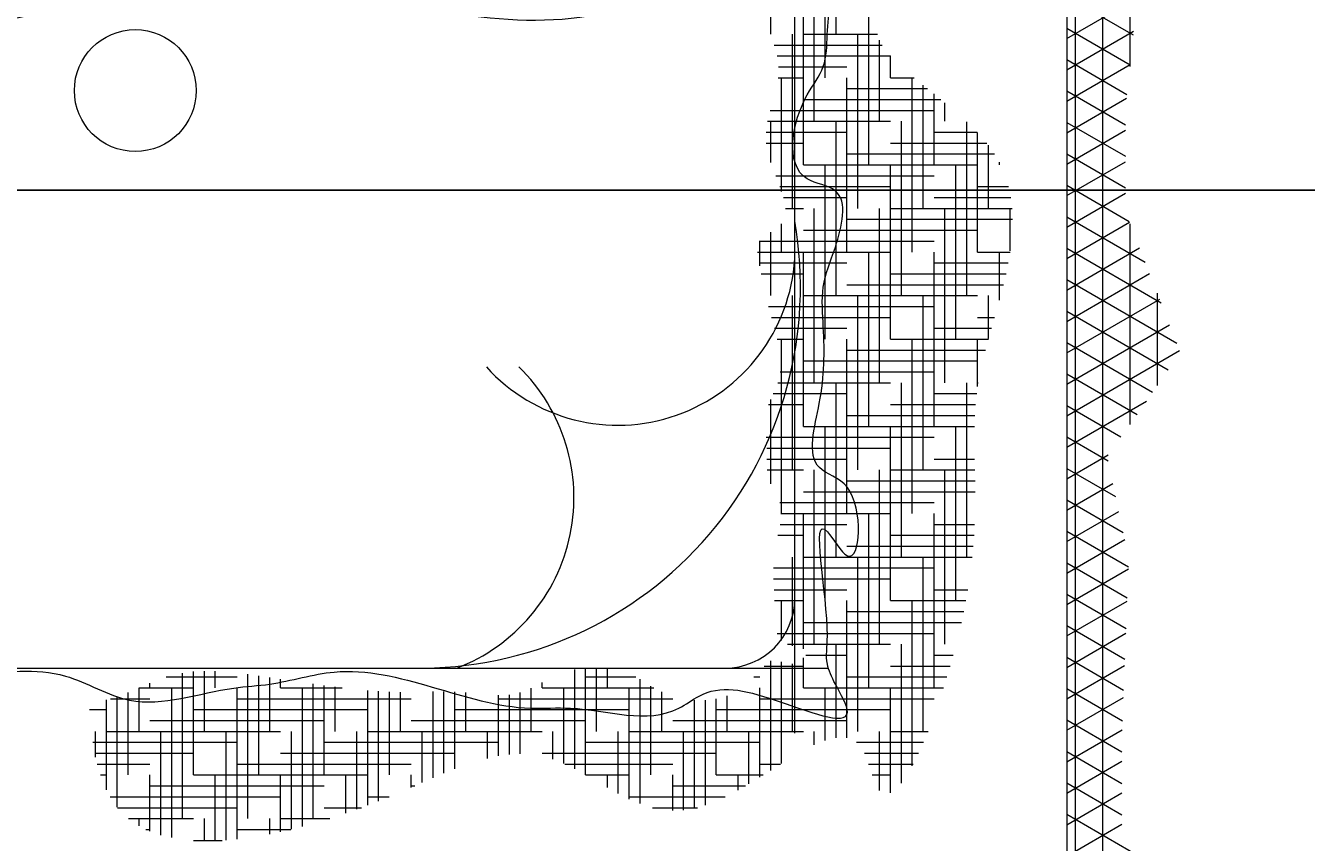
# Model space of a CAD drawing. Units: inches. Extents: x 3731 to 4318, y 1310 to 2388.
# Tile 27 of 57: x 3894 to 3954, y 1844 to 1882. Entities that reach past the tile are written whole.
import ezdxf

# ---------------------------------------------------------------- set-up
doc = ezdxf.new("R2010")
doc.units = ezdxf.units.IN
doc.layers.add('A-ANNO-DIMS', color=2, linetype='Continuous', lineweight=18)
doc.layers.add('A-FURN', color=8, linetype='Continuous', lineweight=13)
doc.styles.get("Standard").update_dxf_attribs({"font": 'arial.ttf'})
doc.dimstyles.get("Standard").update_dxf_attribs({"dimtxt": 0.18, "dimasz": 0.18, "dimexe": 0.18, "dimexo": 0.0625, "dimgap": 0.09, "dimtad": 0, "dimtih": 1, "dimtoh": 1, "dimdec": 4, "dimzin": 0, "dimdsep": 46, "dimtxsty": 'Standard', "dimcen": 0.09, "dimadec": 0, "dimazin": 0, "dimtfac": 1, "dimtdec": 4, "dimtofl": 0, "dimtmove": 0, "dimatfit": 3, "dimfxl": 1, "dimtolj": 1, "dimtzin": 0, "dimarcsym": 0})

# ---------------------------------------------------------------- blocks, each defined once
blk = doc.blocks.new('A$C200C7901')
at = {"linetype": 'ByBlock'}
for p, q in [((2.3224, 0.0468), (2.3224, 1.6627)), ((2.3224, 0.0468), (2.3224, 1.6627)), ((2.3537, 0.0056), (2.3537, 1.634)), ((2.3537, 0.0056), (2.3537, 1.634)), ((2.0474, 1.0977), (2.0474, 1.2977)), ((2.0474, 1.0977), (2.0474, 1.2977)), ((2.3849, 1.0607), (2.3849, 1.3013)), ((2.3849, 1.0607), (2.3849, 1.3013)), ((1.9724, 1.0977), (1.9724, 1.2927)), ((1.9724, 1.0977), (1.9724, 1.2927)), ((2.0349, 1.0477), (2.0349, 1.2477)), ((2.0349, 1.0477), (2.0349, 1.2477)), ((2.0099, 0.9477), (2.0099, 1.1477)), ((2.0099, 0.9477), (2.0099, 1.1477)), ((2.0849, 0.9477), (2.0849, 1.1477)), ((2.0849, 0.9477), (2.0849, 1.1477)), ((2.3121, 1.1408), (2.3884, 1.0967)), ((2.3121, 1.1408), (2.3884, 1.0967)), ((2.3121, 1.0928), (2.3915, 1.1386)), ((2.3121, 1.0928), (2.3915, 1.1386)), ((2.3121, 1.1047), (2.3851, 1.0625)), ((2.3121, 1.1047), (2.3851, 1.0625)), ((1.9974, 0.8977), (1.9974, 1.0977)), ((1.9974, 0.8977), (1.9974, 1.0977)), ((2.0099, 1.0977), (2.095, 1.0977)), ((2.0099, 1.0977), (2.095, 1.0977)), ((2.0724, 0.8977), (2.0724, 1.0977)), ((2.0724, 0.8977), (2.0724, 1.0977)), ((2.0974, 0.9977), (2.0974, 1.0909)), ((2.0974, 0.9977), (2.0974, 1.0909)), ((2.3121, 1.0567), (2.3887, 1.1009)), ((2.3121, 1.0567), (2.3887, 1.1009)), ((1.9763, 1.0852), (2.1005, 1.0852)), ((1.9763, 1.0852), (2.1005, 1.0852)), ((1.9799, 1.0727), (2.1099, 1.0727)), ((1.9799, 1.0727), (2.1099, 1.0727)), ((1.9815, 1.0602), (2.0599, 1.0602)), ((1.9815, 1.0602), (2.0599, 1.0602)), ((2.1099, 1.0477), (2.1099, 1.0729)), ((2.1099, 1.0477), (2.1099, 1.0729)), ((2.3121, 1.0686), (2.3813, 1.0286)), ((2.3121, 1.0686), (2.3813, 1.0286)), ((2.3121, 1.0206), (2.3851, 1.0628)), ((2.3121, 1.0206), (2.3851, 1.0628)), ((1.981, 1.0477), (2.0099, 1.0477)), ((1.981, 1.0477), (2.0099, 1.0477)), ((1.9849, 0.9171), (1.9849, 1.0477)), ((1.9849, 0.9171), (1.9849, 1.0477)), ((2.0599, 0.8477), (2.0599, 1.0477)), ((2.0599, 0.8477), (2.0599, 1.0477)), ((2.1099, 1.0477), (2.137, 1.0477)), ((2.1099, 1.0477), (2.137, 1.0477)), ((2.1349, 0.8477), (2.1349, 1.0477)), ((2.1349, 0.8477), (2.1349, 1.0477)), ((2.0599, 1.0352), (2.1523, 1.0352)), ((2.0599, 1.0352), (2.1523, 1.0352)), ((2.1474, 0.8977), (2.1474, 1.0391)), ((2.1474, 0.8977), (2.1474, 1.0391)), ((2.1599, 0.9477), (2.1599, 1.029)), ((2.1599, 0.9477), (2.1599, 1.029)), ((2.3121, 1.0325), (2.3795, 0.9936)), ((2.3121, 1.0325), (2.3795, 0.9936)), ((2.0099, 1.0227), (2.1678, 1.0227)), ((2.0099, 1.0227), (2.1678, 1.0227)), ((2.1724, 0.9977), (2.1724, 1.0189)), ((2.1724, 0.9977), (2.1724, 1.0189)), ((2.3121, 0.9846), (2.3809, 1.0242)), ((2.3121, 0.9846), (2.3809, 1.0242)), ((1.9718, 1.0102), (2.1599, 1.0102)), ((1.9718, 1.0102), (2.1599, 1.0102)), ((1.9671, 0.9852), (2.0599, 0.9852)), ((1.9671, 0.9852), (2.0599, 0.9852)), ((1.9688, 0.9977), (2.1099, 0.9977)), ((1.9688, 0.9977), (2.1099, 0.9977)), ((1.9724, 0.9504), (1.9724, 0.9977)), ((1.9724, 0.9504), (1.9724, 0.9977)), ((2.0474, 0.7977), (2.0474, 0.9977)), ((2.0474, 0.7977), (2.0474, 0.9977)), ((2.1224, 0.7977), (2.1224, 0.9977)), ((2.1224, 0.7977), (2.1224, 0.9977)), ((2.1599, 0.9852), (2.2095, 0.9852)), ((2.1599, 0.9852), (2.2095, 0.9852)), ((2.1974, 0.7977), (2.1974, 0.9972)), ((2.1974, 0.7977), (2.1974, 0.9972)), ((2.3121, 0.9964), (2.3795, 0.9575)), ((2.3121, 0.9964), (2.3795, 0.9575)), ((2.3121, 0.9485), (2.3795, 0.9874)), ((2.3121, 0.9485), (2.3795, 0.9874)), ((1.9672, 0.9727), (2.0099, 0.9727)), ((1.9672, 0.9727), (2.0099, 0.9727)), ((2.1099, 0.9727), (2.2204, 0.9727)), ((2.1099, 0.9727), (2.2204, 0.9727)), ((2.2099, 0.8477), (2.2099, 0.9848)), ((2.2099, 0.8477), (2.2099, 0.9848)), ((2.0599, 0.9602), (2.2294, 0.9602)), ((2.0599, 0.9602), (2.2294, 0.9602)), ((2.2224, 0.8977), (2.2224, 0.9702)), ((2.2224, 0.8977), (2.2224, 0.9702)), ((2.3121, 0.9603), (2.3795, 0.9215)), ((2.3121, 0.9603), (2.3795, 0.9215)), ((2.0099, 0.9477), (2.2099, 0.9477)), ((2.0099, 0.9477), (2.2099, 0.9477)), ((2.0349, 0.7477), (2.0349, 0.9477)), ((2.0349, 0.7477), (2.0349, 0.9477)), ((2.1099, 0.7477), (2.1099, 0.9477)), ((2.1099, 0.7477), (2.1099, 0.9477)), ((2.1849, 0.7477), (2.1849, 0.9477)), ((2.1849, 0.7477), (2.1849, 0.9477)), ((2.2349, 0.9477), (2.2349, 0.9506)), ((2.2349, 0.9477), (2.2349, 0.9506)), ((2.3121, 0.9124), (2.3795, 0.9513)), ((2.3121, 0.9124), (2.3795, 0.9513)), ((1.9781, 0.9352), (2.1599, 0.9352)), ((1.9781, 0.9352), (2.1599, 0.9352)), ((1.9829, 0.9227), (2.1099, 0.9227)), ((1.9829, 0.9227), (2.1099, 0.9227)), ((2.2099, 0.9227), (2.2455, 0.9227)), ((2.2099, 0.9227), (2.2455, 0.9227)), ((2.3121, 0.9243), (2.3838, 0.8829)), ((2.3121, 0.9243), (2.3838, 0.8829)), ((2.3121, 0.8763), (2.3795, 0.9152)), ((2.3121, 0.8763), (2.3795, 0.9152)), ((1.9871, 0.9102), (2.0599, 0.9102)), ((1.9871, 0.9102), (2.0599, 0.9102)), ((1.9894, 0.8977), (2.0099, 0.8977)), ((1.9894, 0.8977), (2.0099, 0.8977)), ((2.0224, 0.6977), (2.0224, 0.8977)), ((2.0224, 0.6977), (2.0224, 0.8977)), ((2.0974, 0.6977), (2.0974, 0.8977)), ((2.0974, 0.6977), (2.0974, 0.8977)), ((2.1099, 0.8977), (2.2496, 0.8977)), ((2.1099, 0.8977), (2.2496, 0.8977)), ((2.1599, 0.9102), (2.2481, 0.9102)), ((2.1599, 0.9102), (2.2481, 0.9102)), ((2.1724, 0.6977), (2.1724, 0.8977)), ((2.1724, 0.6977), (2.1724, 0.8977)), ((2.2474, 0.8489), (2.2474, 0.8977)), ((2.2474, 0.8489), (2.2474, 0.8977)), ((2.0599, 0.8852), (2.2501, 0.8852)), ((2.0599, 0.8852), (2.2501, 0.8852)), ((2.3121, 0.8882), (2.4022, 0.8362)), ((2.3121, 0.8882), (2.4022, 0.8362)), ((1.9724, 0.7977), (1.9724, 0.8703)), ((1.9724, 0.7977), (1.9724, 0.8703)), ((1.9849, 0.8477), (1.9849, 0.88)), ((1.9849, 0.8477), (1.9849, 0.88)), ((2.0099, 0.8727), (2.2099, 0.8727)), ((2.0099, 0.8727), (2.2099, 0.8727)), ((2.3121, 0.8402), (2.3842, 0.8818)), ((2.3121, 0.8402), (2.3842, 0.8818)), ((2.3849, 0.6497), (2.3849, 0.8801)), ((2.3849, 0.6497), (2.3849, 0.8801)), ((1.9599, 0.8317), (1.9599, 0.8604)), ((1.9599, 0.8317), (1.9599, 0.8604)), ((1.9599, 0.8602), (2.1599, 0.8602)), ((1.9599, 0.8602), (2.1599, 0.8602)), ((1.9574, 0.8477), (2.1099, 0.8477)), ((1.9574, 0.8477), (2.1099, 0.8477)), ((2.0099, 0.6477), (2.0099, 0.8477)), ((2.0099, 0.6477), (2.0099, 0.8477)), ((2.0849, 0.6477), (2.0849, 0.8477)), ((2.0849, 0.6477), (2.0849, 0.8477)), ((2.1599, 0.6477), (2.1599, 0.8477)), ((2.1599, 0.6477), (2.1599, 0.8477)), ((2.2099, 0.8477), (2.2472, 0.8477)), ((2.2099, 0.8477), (2.2472, 0.8477)), ((2.2349, 0.7923), (2.2349, 0.8477)), ((2.2349, 0.7923), (2.2349, 0.8477)), ((2.3121, 0.8041), (2.3958, 0.8524)), ((2.3121, 0.8041), (2.3958, 0.8524)), ((2.3121, 0.8521), (2.4205, 0.7895)), ((2.3121, 0.8521), (2.4205, 0.7895)), ((1.9593, 0.8352), (2.0599, 0.8352)), ((1.9593, 0.8352), (2.0599, 0.8352)), ((2.1599, 0.8352), (2.2451, 0.8352)), ((2.1599, 0.8352), (2.2451, 0.8352)), ((1.9615, 0.8227), (2.0099, 0.8227)), ((1.9615, 0.8227), (2.0099, 0.8227)), ((2.0599, 0.8102), (2.2396, 0.8102)), ((2.0599, 0.8102), (2.2396, 0.8102)), ((2.1099, 0.8227), (2.2425, 0.8227)), ((2.1099, 0.8227), (2.2425, 0.8227)), ((2.3121, 0.7681), (2.4073, 0.823)), ((2.3121, 0.7681), (2.4073, 0.823)), ((2.3121, 0.816), (2.4384, 0.7431)), ((2.3121, 0.816), (2.4384, 0.7431)), ((2.0099, 0.7977), (2.2099, 0.7977)), ((2.0099, 0.7977), (2.2099, 0.7977)), ((2.2224, 0.7483), (2.2224, 0.7977)), ((2.2224, 0.7483), (2.2224, 0.7977)), ((2.4162, 0.6946), (2.4162, 0.8006)), ((2.4162, 0.6946), (2.4162, 0.8006)), ((1.9699, 0.7852), (2.1599, 0.7852)), ((1.9699, 0.7852), (2.1599, 0.7852)), ((2.3121, 0.732), (2.4189, 0.7936)), ((2.3121, 0.732), (2.4189, 0.7936)), ((2.3121, 0.7799), (2.4287, 0.7126)), ((2.3121, 0.7799), (2.4287, 0.7126)), ((1.9734, 0.7727), (2.1099, 0.7727)), ((1.9734, 0.7727), (2.1099, 0.7727)), ((2.2099, 0.7727), (2.2294, 0.7727)), ((2.2099, 0.7727), (2.2294, 0.7727)), ((1.9767, 0.7602), (2.0599, 0.7602)), ((1.9767, 0.7602), (2.0599, 0.7602)), ((2.1599, 0.7602), (2.2258, 0.7602)), ((2.1599, 0.7602), (2.2258, 0.7602)), ((2.3121, 0.6959), (2.4303, 0.7641)), ((2.3121, 0.6959), (2.4303, 0.7641)), ((1.9797, 0.7477), (2.0099, 0.7477)), ((1.9797, 0.7477), (2.0099, 0.7477)), ((2.0599, 0.7352), (2.2188, 0.7352)), ((2.0599, 0.7352), (2.2188, 0.7352)), ((2.1099, 0.7477), (2.2222, 0.7477)), ((2.1099, 0.7477), (2.2222, 0.7477)), ((2.2099, 0.6933), (2.2099, 0.7477)), ((2.2099, 0.6933), (2.2099, 0.7477)), ((2.3121, 0.7438), (2.4108, 0.6869)), ((2.3121, 0.7438), (2.4108, 0.6869)), ((2.0099, 0.7227), (2.2099, 0.7227)), ((2.0099, 0.7227), (2.2099, 0.7227)), ((2.3121, 0.6598), (2.4417, 0.7346)), ((2.3121, 0.6598), (2.4417, 0.7346)), ((1.9831, 0.7102), (2.1599, 0.7102)), ((1.9831, 0.7102), (2.1599, 0.7102)), ((2.3121, 0.7078), (2.3929, 0.6611)), ((2.3121, 0.7078), (2.3929, 0.6611)), ((1.9804, 0.6977), (2.1099, 0.6977)), ((1.9804, 0.6977), (2.1099, 0.6977)), ((2.0474, 0.4977), (2.0474, 0.6977)), ((2.0474, 0.4977), (2.0474, 0.6977)), ((2.1224, 0.4977), (2.1224, 0.6977)), ((2.1224, 0.4977), (2.1224, 0.6977)), ((2.1974, 0.4977), (2.1974, 0.6977)), ((2.1974, 0.4977), (2.1974, 0.6977)), ((2.2099, 0.6977), (2.2106, 0.6977)), ((2.2099, 0.6977), (2.2106, 0.6977)), ((1.9724, 0.5818), (1.9724, 0.6786)), ((1.9724, 0.5818), (1.9724, 0.6786)), ((1.9753, 0.6852), (2.0599, 0.6852)), ((1.9753, 0.6852), (2.0599, 0.6852)), ((2.1599, 0.6852), (2.2088, 0.6852)), ((2.1599, 0.6852), (2.2088, 0.6852)), ((2.3121, 0.6237), (2.4036, 0.6765)), ((2.3121, 0.6237), (2.4036, 0.6765)), ((1.97, 0.6727), (2.0099, 0.6727)), ((1.97, 0.6727), (2.0099, 0.6727)), ((2.1099, 0.6727), (2.2075, 0.6727)), ((2.1099, 0.6727), (2.2075, 0.6727)), ((2.3121, 0.6717), (2.3744, 0.6357)), ((2.3121, 0.6717), (2.3744, 0.6357)), ((2.0099, 0.6477), (2.2062, 0.6477)), ((2.0099, 0.6477), (2.2062, 0.6477)), ((2.0349, 0.4477), (2.0349, 0.6477)), ((2.0349, 0.4477), (2.0349, 0.6477)), ((2.0599, 0.6602), (2.2067, 0.6602)), ((2.0599, 0.6602), (2.2067, 0.6602)), ((2.1099, 0.4477), (2.1099, 0.6477)), ((2.1099, 0.4477), (2.1099, 0.6477)), ((2.1849, 0.4477), (2.1849, 0.6477)), ((2.1849, 0.4477), (2.1849, 0.6477)), ((1.9673, 0.6352), (2.1599, 0.6352)), ((1.9673, 0.6352), (2.1599, 0.6352)), ((2.3121, 0.6356), (2.3598, 0.6081)), ((2.3121, 0.6356), (2.3598, 0.6081)), ((1.9678, 0.6227), (2.1099, 0.6227)), ((1.9678, 0.6227), (2.1099, 0.6227)), ((1.9679, 0.6102), (2.0599, 0.6102)), ((1.9679, 0.6102), (2.0599, 0.6102)), ((2.1599, 0.6102), (2.2064, 0.6102)), ((2.1599, 0.6102), (2.2064, 0.6102)), ((2.3121, 0.5876), (2.3598, 0.6151)), ((2.3121, 0.5876), (2.3598, 0.6151)), ((1.9685, 0.5977), (2.0099, 0.5977)), ((1.9685, 0.5977), (2.0099, 0.5977)), ((2.0224, 0.3977), (2.0224, 0.5977)), ((2.0224, 0.3977), (2.0224, 0.5977)), ((2.0974, 0.3977), (2.0974, 0.5977)), ((2.0974, 0.3977), (2.0974, 0.5977)), ((2.1099, 0.5977), (2.2066, 0.5977)), ((2.1099, 0.5977), (2.2066, 0.5977)), ((2.1724, 0.3977), (2.1724, 0.5977)), ((2.1724, 0.3977), (2.1724, 0.5977)), ((2.3121, 0.5995), (2.3682, 0.5671)), ((2.3121, 0.5995), (2.3682, 0.5671)), ((2.0599, 0.5852), (2.2069, 0.5852)), ((2.0599, 0.5852), (2.2069, 0.5852)), ((2.3121, 0.5515), (2.365, 0.5821)), ((2.3121, 0.5515), (2.365, 0.5821)), ((1.9827, 0.5602), (2.1599, 0.5602)), ((1.9827, 0.5602), (2.1599, 0.5602)), ((2.0099, 0.5727), (2.207, 0.5727)), ((2.0099, 0.5727), (2.207, 0.5727)), ((2.3121, 0.5634), (2.3771, 0.5259)), ((2.3121, 0.5634), (2.3771, 0.5259)), ((1.9842, 0.5477), (2.1099, 0.5477)), ((1.9842, 0.5477), (2.1099, 0.5477)), ((2.0099, 0.3923), (2.0099, 0.5477)), ((2.0099, 0.3923), (2.0099, 0.5477)), ((2.0849, 0.3477), (2.0849, 0.5477)), ((2.0849, 0.3477), (2.0849, 0.5477)), ((2.1599, 0.3477), (2.1599, 0.5477)), ((2.1599, 0.3477), (2.1599, 0.5477)), ((2.3121, 0.5155), (2.3719, 0.55)), ((2.3121, 0.5155), (2.3719, 0.55)), ((1.9831, 0.5352), (2.0599, 0.5352)), ((1.9831, 0.5352), (2.0599, 0.5352)), ((2.1599, 0.5352), (2.2065, 0.5352)), ((2.1599, 0.5352), (2.2065, 0.5352)), ((1.9807, 0.5227), (2.0099, 0.5227)), ((1.9807, 0.5227), (2.0099, 0.5227)), ((2.1099, 0.5227), (2.2058, 0.5227)), ((2.1099, 0.5227), (2.2058, 0.5227)), ((2.3121, 0.5273), (2.383, 0.4864)), ((2.3121, 0.5273), (2.383, 0.4864)), ((2.3121, 0.4794), (2.3788, 0.5179)), ((2.3121, 0.4794), (2.3788, 0.5179)), ((2.0599, 0.5102), (2.2049, 0.5102)), ((2.0599, 0.5102), (2.2049, 0.5102)), ((1.9755, 0.4852), (2.1599, 0.4852)), ((1.9755, 0.4852), (2.1599, 0.4852)), ((1.9974, 0.3957), (1.9974, 0.4977)), ((1.9974, 0.3957), (1.9974, 0.4977)), ((2.0099, 0.4977), (2.2038, 0.4977)), ((2.0099, 0.4977), (2.2038, 0.4977)), ((2.0724, 0.2977), (2.0724, 0.4977)), ((2.0724, 0.2977), (2.0724, 0.4977)), ((2.1474, 0.2977), (2.1474, 0.4977)), ((2.1474, 0.2977), (2.1474, 0.4977)), ((2.3121, 0.4912), (2.3817, 0.4511)), ((2.3121, 0.4912), (2.3817, 0.4511)), ((1.9757, 0.4727), (2.1099, 0.4727)), ((1.9757, 0.4727), (2.1099, 0.4727)), ((2.3121, 0.4433), (2.383, 0.4842)), ((2.3121, 0.4433), (2.383, 0.4842)), ((1.9762, 0.4602), (2.0599, 0.4602)), ((1.9762, 0.4602), (2.0599, 0.4602)), ((2.1599, 0.4602), (2.1987, 0.4602)), ((2.1599, 0.4602), (2.1987, 0.4602)), ((1.9768, 0.4477), (2.0099, 0.4477)), ((1.9768, 0.4477), (2.0099, 0.4477)), ((1.9849, 0.402), (1.9849, 0.4477)), ((1.9849, 0.402), (1.9849, 0.4477)), ((2.0599, 0.2903), (2.0599, 0.4477)), ((2.0599, 0.2903), (2.0599, 0.4477)), ((2.1099, 0.4477), (2.1965, 0.4477)), ((2.1099, 0.4477), (2.1965, 0.4477)), ((2.1349, 0.2582), (2.1349, 0.4477)), ((2.1349, 0.2582), (2.1349, 0.4477)), ((2.3121, 0.4552), (2.3803, 0.4158)), ((2.3121, 0.4552), (2.3803, 0.4158)), ((2.3121, 0.4072), (2.3815, 0.4473)), ((2.3121, 0.4072), (2.3815, 0.4473)), ((2.0599, 0.4352), (2.194, 0.4352)), ((2.0599, 0.4352), (2.194, 0.4352)), ((2.0099, 0.4227), (2.1913, 0.4227)), ((2.0099, 0.4227), (2.1913, 0.4227)), ((2.3121, 0.4191), (2.3789, 0.3805)), ((2.3121, 0.4191), (2.3789, 0.3805)), ((1.9797, 0.4102), (2.1599, 0.4102)), ((1.9797, 0.4102), (2.1599, 0.4102)), ((1.9915, 0.3977), (2.1099, 0.3977)), ((1.9915, 0.3977), (2.1099, 0.3977)), ((2.0474, 0.2905), (2.0474, 0.3977)), ((2.0474, 0.2905), (2.0474, 0.3977)), ((2.1224, 0.2385), (2.1224, 0.3977)), ((2.1224, 0.2385), (2.1224, 0.3977)), ((2.3121, 0.3711), (2.3801, 0.4103)), ((2.3121, 0.3711), (2.3801, 0.4103)), ((2.0127, 0.3852), (2.0599, 0.3852)), ((2.0127, 0.3852), (2.0599, 0.3852)), ((2.1599, 0.3852), (2.1819, 0.3852)), ((2.1599, 0.3852), (2.1819, 0.3852)), ((2.3121, 0.383), (2.3775, 0.3452)), ((2.3121, 0.383), (2.3775, 0.3452)), ((1.7474, 0.2546), (1.7474, 0.3689)), ((1.7474, 0.2546), (1.7474, 0.3689)), ((1.7599, 0.2477), (1.7599, 0.3703)), ((1.7599, 0.2477), (1.7599, 0.3703)), ((1.7724, 0.2977), (1.7724, 0.3703)), ((1.7724, 0.2977), (1.7724, 0.3703)), ((1.7849, 0.3477), (1.7849, 0.3703)), ((1.7849, 0.3477), (1.7849, 0.3703)), ((1.9648, 0.3727), (2.0099, 0.3727)), ((1.9648, 0.3727), (2.0099, 0.3727)), ((1.9724, 0.253), (1.9724, 0.3785)), ((1.9724, 0.253), (1.9724, 0.3785)), ((1.9849, 0.2609), (1.9849, 0.3774)), ((1.9849, 0.2609), (1.9849, 0.3774)), ((1.9974, 0.2977), (1.9974, 0.3753)), ((1.9974, 0.2977), (1.9974, 0.3753)), ((2.0099, 0.3477), (2.0099, 0.382)), ((2.0099, 0.3477), (2.0099, 0.382)), ((2.1099, 0.3727), (2.1784, 0.3727)), ((2.1099, 0.3727), (2.1784, 0.3727)), ((2.3121, 0.335), (2.3786, 0.3734)), ((2.3121, 0.335), (2.3786, 0.3734)), ((1.2599, 0.3477), (1.2599, 0.3531)), ((1.2599, 0.3477), (1.2599, 0.3531)), ((1.2785, 0.3602), (1.3599, 0.3602)), ((1.2785, 0.3602), (1.3599, 0.3602)), ((1.2974, 0.1977), (1.2974, 0.3647)), ((1.2974, 0.1977), (1.2974, 0.3647)), ((1.3099, 0.2477), (1.3099, 0.3663)), ((1.3099, 0.2477), (1.3099, 0.3663)), ((1.3224, 0.2977), (1.3224, 0.3669)), ((1.3224, 0.2977), (1.3224, 0.3669)), ((1.3349, 0.3477), (1.3349, 0.3668)), ((1.3349, 0.3477), (1.3349, 0.3668)), ((1.3724, 0.1977), (1.3724, 0.3634)), ((1.3724, 0.1977), (1.3724, 0.3634)), ((1.3849, 0.2477), (1.3849, 0.3616)), ((1.3849, 0.2477), (1.3849, 0.3616)), ((1.3974, 0.2977), (1.3974, 0.3597)), ((1.3974, 0.2977), (1.3974, 0.3597)), ((1.4099, 0.3477), (1.4099, 0.3578)), ((1.4099, 0.3477), (1.4099, 0.3578)), ((1.7099, 0.3477), (1.7099, 0.3539)), ((1.7099, 0.3477), (1.7099, 0.3539)), ((1.7599, 0.3602), (1.8177, 0.3602)), ((1.7599, 0.3602), (1.8177, 0.3602)), ((1.8224, 0.2148), (1.8224, 0.3575)), ((1.8224, 0.2148), (1.8224, 0.3575)), ((1.9532, 0.3602), (1.9599, 0.3602)), ((1.9532, 0.3602), (1.9599, 0.3602)), ((2.0599, 0.3602), (2.1747, 0.3602)), ((2.0599, 0.3602), (2.1747, 0.3602)), ((1.2349, 0.2477), (1.2349, 0.3422)), ((1.2349, 0.2477), (1.2349, 0.3422)), ((1.2474, 0.2977), (1.2474, 0.3476)), ((1.2474, 0.2977), (1.2474, 0.3476)), ((1.2475, 0.3477), (1.3099, 0.3477)), ((1.2475, 0.3477), (1.3099, 0.3477)), ((1.2849, 0.1758), (1.2849, 0.3477)), ((1.2849, 0.1758), (1.2849, 0.3477)), ((1.3599, 0.1741), (1.3599, 0.3477)), ((1.3599, 0.1741), (1.3599, 0.3477)), ((1.4099, 0.3477), (1.4806, 0.3477)), ((1.4099, 0.3477), (1.4806, 0.3477)), ((1.4349, 0.1886), (1.4349, 0.3477)), ((1.4349, 0.1886), (1.4349, 0.3477)), ((1.4474, 0.1977), (1.4474, 0.3521)), ((1.4474, 0.1977), (1.4474, 0.3521)), ((1.4599, 0.2477), (1.4599, 0.3504)), ((1.4599, 0.2477), (1.4599, 0.3504)), ((1.4724, 0.2977), (1.4724, 0.3487)), ((1.4724, 0.2977), (1.4724, 0.3487)), ((1.5099, 0.2129), (1.5099, 0.3447)), ((1.5099, 0.2129), (1.5099, 0.3447)), ((1.5224, 0.2177), (1.5224, 0.3438)), ((1.5224, 0.2177), (1.5224, 0.3438)), ((1.5349, 0.2477), (1.5349, 0.3431)), ((1.5349, 0.2477), (1.5349, 0.3431)), ((1.5474, 0.2977), (1.5474, 0.3428)), ((1.5474, 0.2977), (1.5474, 0.3428)), ((1.5849, 0.2443), (1.5849, 0.3434)), ((1.5849, 0.2443), (1.5849, 0.3434)), ((1.5974, 0.2496), (1.5974, 0.3435)), ((1.5974, 0.2496), (1.5974, 0.3435)), ((1.6099, 0.2546), (1.6099, 0.3432)), ((1.6099, 0.2546), (1.6099, 0.3432)), ((1.6224, 0.2977), (1.6224, 0.3424)), ((1.6224, 0.2977), (1.6224, 0.3424)), ((1.6599, 0.2695), (1.6599, 0.3394)), ((1.6599, 0.2695), (1.6599, 0.3394)), ((1.6724, 0.2713), (1.6724, 0.3398)), ((1.6724, 0.2713), (1.6724, 0.3398)), ((1.6849, 0.272), (1.6849, 0.3422)), ((1.6849, 0.272), (1.6849, 0.3422)), ((1.6974, 0.2977), (1.6974, 0.3472)), ((1.6974, 0.2977), (1.6974, 0.3472)), ((1.7099, 0.3477), (1.8383, 0.3477)), ((1.7099, 0.3477), (1.8383, 0.3477)), ((1.7349, 0.2607), (1.7349, 0.3477)), ((1.7349, 0.2607), (1.7349, 0.3477)), ((1.8099, 0.2201), (1.8099, 0.3477)), ((1.8099, 0.2201), (1.8099, 0.3477)), ((1.8349, 0.2477), (1.8349, 0.3497)), ((1.8349, 0.2477), (1.8349, 0.3497)), ((1.8474, 0.2977), (1.8474, 0.3432)), ((1.8474, 0.2977), (1.8474, 0.3432)), ((1.9224, 0.2977), (1.9224, 0.3385)), ((1.9224, 0.2977), (1.9224, 0.3385)), ((1.9599, 0.2452), (1.9599, 0.3477)), ((1.9599, 0.2452), (1.9599, 0.3477)), ((2.0099, 0.3477), (2.1708, 0.3477)), ((2.0099, 0.3477), (2.1708, 0.3477)), ((2.0349, 0.2874), (2.0349, 0.3477)), ((2.0349, 0.2874), (2.0349, 0.3477)), ((2.1099, 0.2274), (2.1099, 0.3477)), ((2.1099, 0.2274), (2.1099, 0.3477)), ((2.3121, 0.3469), (2.3761, 0.31)), ((2.3121, 0.3469), (2.3761, 0.31)), ((1.2099, 0.2308), (1.2099, 0.334)), ((1.2099, 0.2308), (1.2099, 0.334)), ((1.2148, 0.3352), (1.2599, 0.3352)), ((1.2148, 0.3352), (1.2599, 0.3352)), ((1.2224, 0.2106), (1.2224, 0.3375)), ((1.2224, 0.2106), (1.2224, 0.3375)), ((1.3599, 0.3352), (1.5599, 0.3352)), ((1.3599, 0.3352), (1.5599, 0.3352)), ((1.6599, 0.3352), (1.8599, 0.3352)), ((1.6599, 0.3352), (1.8599, 0.3352)), ((1.8849, 0.2093), (1.8849, 0.3337)), ((1.8849, 0.2093), (1.8849, 0.3337)), ((1.8974, 0.2129), (1.8974, 0.3335)), ((1.8974, 0.2129), (1.8974, 0.3335)), ((1.9099, 0.2477), (1.9099, 0.3349)), ((1.9099, 0.2477), (1.9099, 0.3349)), ((1.9599, 0.3352), (2.1599, 0.3352)), ((1.9599, 0.3352), (2.1599, 0.3352)), ((2.3121, 0.299), (2.3772, 0.3365)), ((2.3121, 0.299), (2.3772, 0.3365)), ((1.1904, 0.3227), (1.2099, 0.3227)), ((1.1904, 0.3227), (1.2099, 0.3227)), ((1.2599, 0.3102), (1.4599, 0.3102)), ((1.2599, 0.3102), (1.4599, 0.3102)), ((1.3099, 0.3227), (1.5099, 0.3227)), ((1.3099, 0.3227), (1.5099, 0.3227)), ((1.5599, 0.3102), (1.7599, 0.3102)), ((1.5599, 0.3102), (1.7599, 0.3102)), ((1.6099, 0.3227), (1.8099, 0.3227)), ((1.6099, 0.3227), (1.8099, 0.3227)), ((1.8599, 0.3102), (2.0599, 0.3102)), ((1.8599, 0.3102), (2.0599, 0.3102)), ((1.9099, 0.3227), (2.1099, 0.3227)), ((1.9099, 0.3227), (2.1099, 0.3227)), ((2.3121, 0.3108), (2.3755, 0.2742)), ((2.3121, 0.3108), (2.3755, 0.2742)), ((1.1974, 0.2683), (1.1974, 0.2977)), ((1.1974, 0.2683), (1.1974, 0.2977)), ((1.2099, 0.2977), (1.4099, 0.2977)), ((1.2099, 0.2977), (1.4099, 0.2977)), ((1.2724, 0.1788), (1.2724, 0.2977)), ((1.2724, 0.1788), (1.2724, 0.2977)), ((1.3474, 0.173), (1.3474, 0.2977)), ((1.3474, 0.173), (1.3474, 0.2977)), ((1.4224, 0.1854), (1.4224, 0.2977)), ((1.4224, 0.1854), (1.4224, 0.2977)), ((1.4974, 0.2083), (1.4974, 0.2977)), ((1.4974, 0.2083), (1.4974, 0.2977)), ((1.5099, 0.2977), (1.7099, 0.2977)), ((1.5099, 0.2977), (1.7099, 0.2977)), ((1.5724, 0.2389), (1.5724, 0.2977)), ((1.5724, 0.2389), (1.5724, 0.2977)), ((1.6474, 0.2668), (1.6474, 0.2977)), ((1.6474, 0.2668), (1.6474, 0.2977)), ((1.7224, 0.2658), (1.7224, 0.2977)), ((1.7224, 0.2658), (1.7224, 0.2977)), ((1.7974, 0.2263), (1.7974, 0.2977)), ((1.7974, 0.2263), (1.7974, 0.2977)), ((1.8099, 0.2977), (2.0099, 0.2977)), ((1.8099, 0.2977), (2.0099, 0.2977)), ((1.8724, 0.2072), (1.8724, 0.2977)), ((1.8724, 0.2072), (1.8724, 0.2977)), ((1.9474, 0.2376), (1.9474, 0.2977)), ((1.9474, 0.2376), (1.9474, 0.2977)), ((2.0224, 0.2822), (2.0224, 0.2977)), ((2.0224, 0.2822), (2.0224, 0.2977)), ((2.0974, 0.2299), (2.0974, 0.2977)), ((2.0974, 0.2299), (2.0974, 0.2977)), ((2.1099, 0.2977), (2.153, 0.2977)), ((2.1099, 0.2977), (2.153, 0.2977)), ((2.3121, 0.2629), (2.3757, 0.2996)), ((2.3121, 0.2629), (2.3757, 0.2996)), ((1.1943, 0.2852), (1.3599, 0.2852)), ((1.1943, 0.2852), (1.3599, 0.2852)), ((1.4599, 0.2852), (1.6599, 0.2852)), ((1.4599, 0.2852), (1.6599, 0.2852)), ((1.7599, 0.2852), (1.9599, 0.2852)), ((1.7599, 0.2852), (1.9599, 0.2852)), ((2.0708, 0.2852), (2.1478, 0.2852)), ((2.0708, 0.2852), (2.1478, 0.2852)), ((1.1965, 0.2727), (1.3099, 0.2727)), ((1.1965, 0.2727), (1.3099, 0.2727)), ((1.4099, 0.2727), (1.6099, 0.2727)), ((1.4099, 0.2727), (1.6099, 0.2727)), ((1.7099, 0.2727), (1.9099, 0.2727)), ((1.7099, 0.2727), (1.9099, 0.2727)), ((2.08, 0.2727), (2.1422, 0.2727)), ((2.08, 0.2727), (2.1422, 0.2727)), ((2.3121, 0.2747), (2.3755, 0.2381)), ((2.3121, 0.2747), (2.3755, 0.2381)), ((1.1994, 0.2602), (1.2599, 0.2602)), ((1.1994, 0.2602), (1.2599, 0.2602)), ((1.3599, 0.2602), (1.5599, 0.2602)), ((1.3599, 0.2602), (1.5599, 0.2602)), ((1.7361, 0.2602), (1.8599, 0.2602)), ((1.7361, 0.2602), (1.8599, 0.2602)), ((1.9599, 0.2602), (1.9838, 0.2602)), ((1.9599, 0.2602), (1.9838, 0.2602)), ((2.0848, 0.2602), (2.1359, 0.2602)), ((2.0848, 0.2602), (2.1359, 0.2602)), ((2.3121, 0.2268), (2.3755, 0.2634)), ((2.3121, 0.2268), (2.3755, 0.2634)), ((1.2031, 0.2477), (1.2099, 0.2477)), ((1.2031, 0.2477), (1.2099, 0.2477)), ((1.2599, 0.1831), (1.2599, 0.2477)), ((1.2599, 0.1831), (1.2599, 0.2477)), ((1.3099, 0.2477), (1.5099, 0.2477)), ((1.3099, 0.2477), (1.5099, 0.2477)), ((1.3349, 0.1723), (1.3349, 0.2477)), ((1.3349, 0.1723), (1.3349, 0.2477)), ((1.4099, 0.1825), (1.4099, 0.2477)), ((1.4099, 0.1825), (1.4099, 0.2477)), ((1.4849, 0.2039), (1.4849, 0.2477)), ((1.4849, 0.2039), (1.4849, 0.2477)), ((1.5599, 0.2335), (1.5599, 0.2477)), ((1.5599, 0.2335), (1.5599, 0.2477)), ((1.7599, 0.2477), (1.8099, 0.2477)), ((1.7599, 0.2477), (1.8099, 0.2477)), ((1.7849, 0.2332), (1.7849, 0.2477)), ((1.7849, 0.2332), (1.7849, 0.2477)), ((1.8599, 0.2068), (1.8599, 0.2477)), ((1.8599, 0.2068), (1.8599, 0.2477)), ((1.9099, 0.2477), (1.9639, 0.2477)), ((1.9099, 0.2477), (1.9639, 0.2477)), ((1.9349, 0.2304), (1.9349, 0.2477)), ((1.9349, 0.2304), (1.9349, 0.2477)), ((2.0888, 0.2477), (2.1099, 0.2477)), ((2.0888, 0.2477), (2.1099, 0.2477)), ((2.3121, 0.2387), (2.3755, 0.202)), ((2.3121, 0.2387), (2.3755, 0.202)), ((1.2142, 0.2227), (1.4099, 0.2227)), ((1.2142, 0.2227), (1.4099, 0.2227)), ((1.2599, 0.2352), (1.4599, 0.2352)), ((1.2599, 0.2352), (1.4599, 0.2352)), ((1.5099, 0.2227), (1.5346, 0.2227)), ((1.5099, 0.2227), (1.5346, 0.2227)), ((1.5599, 0.2352), (1.5638, 0.2352)), ((1.5599, 0.2352), (1.5638, 0.2352)), ((1.8099, 0.2227), (1.9203, 0.2227)), ((1.8099, 0.2227), (1.9203, 0.2227)), ((1.8599, 0.2352), (1.9433, 0.2352)), ((1.8599, 0.2352), (1.9433, 0.2352)), ((2.3121, 0.1907), (2.3755, 0.2273)), ((2.3121, 0.1907), (2.3755, 0.2273)), ((1.2227, 0.2102), (1.3599, 0.2102)), ((1.2227, 0.2102), (1.3599, 0.2102)), ((1.4599, 0.2102), (1.5027, 0.2102)), ((1.4599, 0.2102), (1.5027, 0.2102)), ((1.8368, 0.2102), (1.8884, 0.2102)), ((1.8368, 0.2102), (1.8884, 0.2102)), ((1.2351, 0.1977), (1.3099, 0.1977)), ((1.2351, 0.1977), (1.3099, 0.1977)), ((1.2474, 0.1892), (1.2474, 0.1977)), ((1.2474, 0.1892), (1.2474, 0.1977)), ((1.3224, 0.1722), (1.3224, 0.1977)), ((1.3224, 0.1722), (1.3224, 0.1977)), ((1.3974, 0.1799), (1.3974, 0.1977)), ((1.3974, 0.1799), (1.3974, 0.1977)), ((1.4099, 0.1977), (1.4662, 0.1977)), ((1.4099, 0.1977), (1.4662, 0.1977)), ((2.3121, 0.2026), (2.3953, 0.1545)), ((2.3121, 0.2026), (2.3953, 0.1545)), ((2.3121, 0.1546), (2.3755, 0.1912)), ((2.3121, 0.1546), (2.3755, 0.1912)), ((1.2552, 0.1852), (1.2599, 0.1852)), ((1.2552, 0.1852), (1.2599, 0.1852)), ((1.3599, 0.1852), (1.4215, 0.1852)), ((1.3599, 0.1852), (1.4215, 0.1852)), ((1.3099, 0.1727), (1.3428, 0.1727)), ((1.3099, 0.1727), (1.3428, 0.1727))]:
    blk.add_line(p, q, dxfattribs=at)
for p, q in [((2.3121, 1.6596), (2.3121, 0.0201)), ((2, 0.2957), (2, 1.2957)), ((2.0224, 0.9977), (2.0224, 1.1977)), ((2.0224, 0.9977), (2.0224, 1.1977)), ((1.9974, 0.5977), (1.9974, 0.7977)), ((1.9974, 0.5977), (1.9974, 0.7977)), ((2.0724, 0.5977), (2.0724, 0.7977)), ((2.0724, 0.5977), (2.0724, 0.7977)), ((2.1474, 0.5977), (2.1474, 0.7977)), ((2.1474, 0.5977), (2.1474, 0.7977)), ((1.9849, 0.5477), (1.9849, 0.7477)), ((1.9849, 0.5477), (1.9849, 0.7477)), ((2.0599, 0.5477), (2.0599, 0.7477)), ((2.0599, 0.5477), (2.0599, 0.7477)), ((2.1349, 0.5477), (2.1349, 0.7477)), ((2.1349, 0.5477), (2.1349, 0.7477)), ((0.4061, 0.3703), (2.0386, 0.3703))]:
    blk.add_line(p, q)
blk.add_circle((1.2431, 1.0329), 0.0699)
for centre, radius, start, end in [((1.5693, 0.8075), 0.4372, 269.0679, 9.9322), ((1.7969, 0.8525), 0.2035, 222.1514, 356.4639), ((1.5372, 0.5659), 0.2094, 290.9415, 45.7647), ((1.92, 0.4503), 0.08, 270, 0)]:
    blk.add_arc(centre, radius, start, end)
blk.add_open_spline([(0.4856, 1.3429), (0.5504, 1.3182), (0.6715, 1.2721), (0.8374, 1.0498), (1.1164, 1.1183), (1.3878, 1.1816), (1.5888, 1.1102), (1.8403, 1.1127), (1.9415, 1.2178), (2.0032, 1.2819)], degree=3, knots=[0, 0, 0, 0, 205.411753, 383.654933, 772.067458, 921.644661, 1226.793228, 1388.983508, 1642.292305, 1642.292305, 1642.292305, 1642.292305])
blk.add_open_spline([(0.473, 1.2954), (0.4739, 1.2781), (0.4755, 1.2477), (0.5032, 1.2084), (0.4801, 1.1701), (0.4928, 1.1255), (0.4674, 1.0912), (0.4579, 1.0351), (0.501, 0.9724), (0.4311, 0.8832), (0.4902, 0.8637), (0.4843, 0.8288), (0.4774, 0.7906), (0.4625, 0.7457), (0.459, 0.6999), (0.4816, 0.6664), (0.4748, 0.625), (0.4791, 0.5889), (0.4533, 0.5528), (0.4738, 0.5004), (0.4658, 0.4502), (0.4696, 0.3946), (0.4189, 0.3935), (0.4493, 0.3684), (0.4694, 0.3857), (0.4922, 0.3576), (0.5297, 0.3262), (0.5917, 0.3353), (0.6454, 0.3754), (0.7083, 0.3741), (0.7643, 0.3328), (0.826, 0.346), (0.925, 0.3388), (1.0353, 0.3593), (1.1561, 0.3744), (1.2477, 0.3154), (1.3302, 0.3474), (1.4086, 0.3512), (1.5217, 0.3878), (1.6362, 0.3176), (1.7682, 0.3285), (1.8402, 0.3019), (1.9071, 0.3529), (1.9647, 0.3412), (2.0795, 0.2948), (2.0472, 0.3498), (2.0343, 0.3772), (2.0435, 0.43), (2.0109, 0.5782), (2.0746, 0.4643), (2.0805, 0.584), (2.0084, 0.5979), (2.0343, 0.6846), (2.0344, 0.746), (2.0293, 0.8096), (2.0489, 0.8545), (2.0652, 0.9218), (1.9842, 0.9297), (2.0007, 1.0162), (2.0367, 1.0585), (2.0367, 1.1102), (2.0457, 1.1647), (2.0226, 1.2084), (2.0234, 1.2306), (2.0236, 1.2352)], degree=3, knots=[0, 0, 0, 0, 51.660678, 90.967412, 128.902454, 170.303599, 219.852997, 247.834962, 336.321557, 429.35469, 458.821847, 477.222321, 524.135809, 581.038434, 617.839381, 657.146115, 693.947125, 740.178081, 760.753248, 820.731705, 885.133458, 928.777044, 953.563729, 976.574207, 995.553042, 1018.563482, 1064.584401, 1147.951297, 1174.787598, 1266.851571, 1308.018447, 1377.066427, 1441.511314, 1608.245014, 1714.11869, 1792.771707, 1913.247991, 1954.931389, 2029.864445, 2259.189419, 2305.221512, 2429.507982, 2456.344283, 2543.92595, 2627.925037, 2662.96218, 2687.736879, 2719.937755, 2839.540991, 2875.47895, 2953.681041, 2993.270313, 3066.872333, 3154.395764, 3200.397042, 3248.426375, 3312.828127, 3347.881398, 3444.484026, 3481.577522, 3518.665244, 3592.267265, 3644.719162, 3658.519501, 3658.519501, 3658.519501, 3658.519501], dxfattribs=at)
blk = doc.blocks.new('*D45')
at = {"layer": 'A-ANNO-DIMS', "color": 0, "lineweight": -2, "transparency": 16777216}
for p, q in [((3969.146, 1934.382), (3731.412, 1934.382)), ((3731.592, 1934.202), (3731.592, 1904.563)), ((3731.592, 1874.562), (3731.592, 1904.2)), ((3969.146, 1874.382), (3731.412, 1874.382))]:
    blk.add_line(p, q, dxfattribs=at)
at = {"layer": 'A-ANNO-DIMS', "color": 0, "transparency": 16777216}
for points in [[(3731.562, 1934.202), (3731.622, 1934.202), (3731.592, 1934.382)], [(3731.562, 1874.562), (3731.622, 1874.562), (3731.592, 1874.382)]]:
    blk.add_solid(points, dxfattribs=at)
at = {"layer": 'Defpoints', "color": 0, "transparency": 16777216}
for p in [(3731.592, 1934.382), (3969.209, 1934.382), (3969.209, 1874.382)]:
    blk.add_point(p, dxfattribs=at)
at = {"layer": 'A-ANNO-DIMS', "color": 0, "transparency": 16777216, "insert": (3731.592, 1904.382), "char_height": 0.18, "attachment_point": 5}
blk.add_mtext('\\A1;60', dxfattribs=at)

msp = doc.modelspace()

# ---------------------------------------------------------------- block references
at = {"layer": 'A-FURN', "xscale": 41.1071563136412, "yscale": 41.1071563136412, "zscale": 41.1071563136412}
msp.add_blockref('A$C200C7901', (3848.004, 1836.625), dxfattribs=at)

# ---------------------------------------------------------------- dimensions: what is measured, and where the dimension line sits
at = {"layer": 'A-ANNO-DIMS'}
dim = msp.add_linear_dim(base=(3731.592, 1934.382), p1=(3969.209, 1874.382), p2=(3969.209, 1934.382), angle=90, dimstyle='Standard', override={"dimdec": 0, "dimlfac": 1, "dimrnd": 0, "dimzin": 0, "dimdsep": 46, "dimlunit": 2}, dxfattribs=at)
dim.commit()
dim.dimension.update_dxf_attribs({"geometry": '*D45', "text_midpoint": (3731.592, 1904.382)})

doc.saveas('drawing.dxf')
